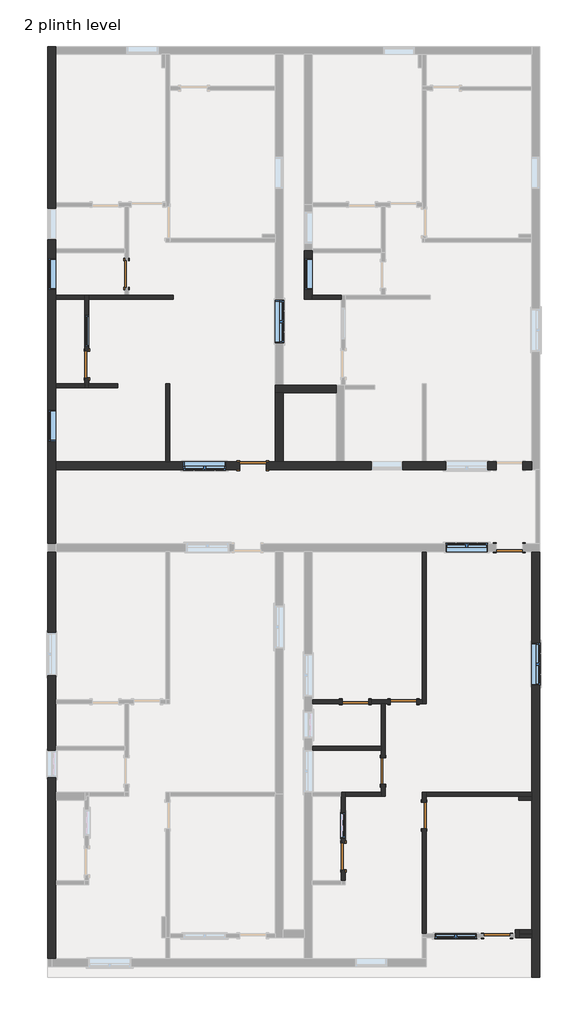
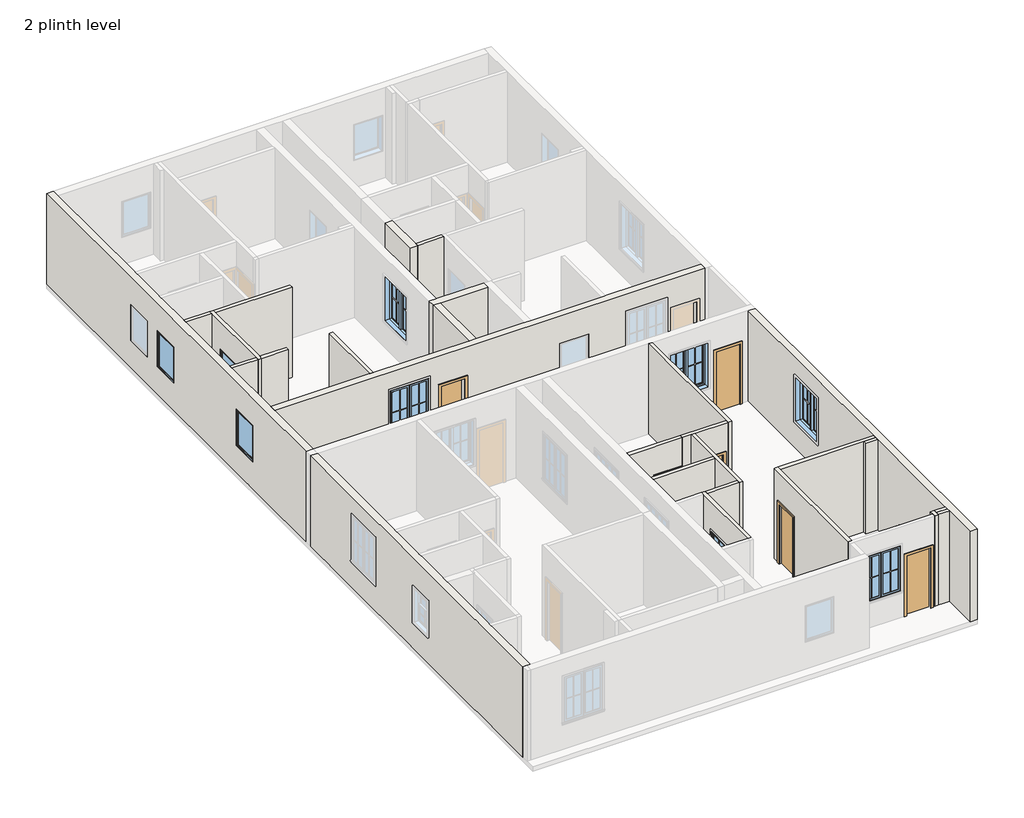
# One storey, part 2 of 4: 27 walls, 10 doors, 10 windows.
"""IFC4 building model written with IfcOpenShell, lengths in millimetres."""

from ifc_helpers import new_model, si_unit, frame, origin, place, context, project, spatial, polyline, outline, extrude, faceted_brep, transform, mapped, element, save
from components import door_d8f5dbb5, door_a1484949, door_f2b275c1, door_85036156, window_c1f32544, window_41a96561, window_8377141f, window_d9d3dda5, window_5a369d27

model = new_model("IFC4")

# Units and contexts
model_context = context("Model", 3, world=origin())
ifc_project = project(units=[si_unit("LENGTHUNIT", "METRE", prefix="MILLI")], contexts=[model_context])

# Site, building, storey
site = spatial("IfcSite", under=ifc_project)
building = spatial("IfcBuilding", under=site)
storey = spatial("IfcBuildingStorey", under=building, Name="2 plinth level", Elevation=457.2)

# Doors
placement = place(None, origin())
door_shape = door_d8f5dbb5(model_context)
element("IfcDoor", 1, ObjectType="Single-Flush : 30\" x 80\"", at=placement, inside=storey, context=model_context, shape_type="MappedRepresentation", body=[
    mapped(door_shape, transform((4590.996455, -11604.0784449, 457.2), x_axis=(1.0, 0.0, 0.0), y_axis=(0.0, 1.0, 0.0), z_axis=(0.0, 0.0, 1.0))),
])
element("IfcDoor", 2, ObjectType="Single-Flush : 30\" x 80\"", at=placement, inside=storey, context=model_context, shape_type="MappedRepresentation", body=[
    mapped(door_shape, transform((1896.0224532, -4857.3304449, 457.2), x_axis=(1.0, 0.0, 0.0), y_axis=(0.0, 1.0, 0.0), z_axis=(0.0, 0.0, 1.0))),
])
door_2_shape = door_a1484949(model_context)
element("IfcDoor", 3, ObjectType="Single-Flush : 30\" x 80\"", at=placement, inside=storey, context=model_context, shape_type="MappedRepresentation", body=[
    mapped(door_2_shape, transform((-2447.3775468, 1943.5195552, 457.2), x_axis=(1.0, 0.0, 0.0), y_axis=(0.0, 1.0, 0.0), z_axis=(0.0, 0.0, 1.0))),
])
door_3_shape = door_f2b275c1(model_context)
element("IfcDoor", 4, ObjectType="Single-Flush : 30\" x 80\"", at=placement, inside=storey, context=model_context, shape_type="MappedRepresentation", body=[
    mapped(door_3_shape, transform((-6085.9275468, 7468.0195551, 457.2), x_axis=(0.0, -1.0, 0.0), y_axis=(1.0, 0.0, 0.0), z_axis=(0.0, 0.0, 1.0))),
])
element("IfcDoor", 5, ObjectType="Single-Flush : 30\" x 80\"", at=placement, inside=storey, context=model_context, shape_type="MappedRepresentation", body=[
    mapped(door_3_shape, transform((-7228.9275468, 4858.1695551, 457.2), x_axis=(0.0, -1.0, 0.0), y_axis=(1.0, 0.0, 0.0), z_axis=(0.0, 0.0, 1.0))),
])
element("IfcDoor", 6, ObjectType="Single-Flush : 30\" x 80\"", at=placement, inside=storey, context=model_context, shape_type="MappedRepresentation", body=[
    mapped(door_3_shape, transform((505.5435023, -4857.3304449, 457.2), x_axis=(1.0, 0.0, 0.0), y_axis=(0.0, 1.0, 0.0), z_axis=(0.0, 0.0, 1.0))),
])
element("IfcDoor", 7, ObjectType="Single-Flush : 30\" x 80\"", at=placement, inside=storey, context=model_context, shape_type="MappedRepresentation", body=[
    mapped(door_3_shape, transform((1305.4724532, -6857.5804449, 457.2), x_axis=(0.0, -1.0, 0.0), y_axis=(1.0, 0.0, 0.0), z_axis=(0.0, 0.0, 1.0))),
])
element("IfcDoor", 8, ObjectType="Single-Flush : 30\" x 80\"", at=placement, inside=storey, context=model_context, shape_type="MappedRepresentation", body=[
    mapped(door_3_shape, transform((162.4724532, -9315.0304449, 457.2), x_axis=(0.0, -1.0, 0.0), y_axis=(1.0, 0.0, 0.0), z_axis=(0.0, 0.0, 1.0))),
])
element("IfcDoor", 9, ObjectType="Single-Flush : 30\" x 80\"", at=placement, inside=storey, context=model_context, shape_type="MappedRepresentation", body=[
    mapped(door_3_shape, transform((2486.5724532, -8133.9304449, 457.2), x_axis=(0.0, 1.0, 0.0), y_axis=(-1.0, 0.0, 0.0), z_axis=(0.0, 0.0, 1.0))),
])
door_4_shape = door_85036156(model_context)
element("IfcDoor", 10, ObjectType="Single-Flush : 30\" x 80\"", at=placement, inside=storey, context=model_context, shape_type="MappedRepresentation", body=[
    mapped(door_4_shape, transform((4944.0224532, -418.6804449, 457.2), x_axis=(1.0, 0.0, 0.0), y_axis=(0.0, 1.0, 0.0), z_axis=(0.0, 0.0, 1.0))),
])

# Walls
element("IfcWall", 11, ObjectType="4.5\"", at=placement, inside=storey, context=model_context, shape_type="SweptSolid", body=[
    extrude(outline(polyline([(-7286.0775468, 6744.1195551), (-8124.2775468, 6744.1195551), (-8124.2775468, 6858.4195551), (-7286.0775468, 6858.4195551), (-7286.0775468, 6744.1195551)])), frame((0.0, 0.0, 457.2), z_axis=(0.0, 0.0, 1.0), x_axis=(1.0, 0.0, 0.0)), (0.0, 0.0, 1.0), 3048.0),
])
element("IfcWall", 12, ObjectType="4.5\"", at=placement, inside=storey, context=model_context, shape_type="Brep", body=[
    faceted_brep([(-7171.7775468, 6744.1195551, 457.2), (-4733.3775468, 6744.1195551, 457.2), (-4733.3775468, 6744.1195551, 3505.2), (-7171.7775468, 6744.1195551, 3505.2), (-7171.7775468, 6858.4195551, 457.2), (-7171.7775468, 6858.4195551, 3505.2), (-6143.0775468, 6858.4195551, 3505.2), (-6028.7775468, 6858.4195551, 3505.2), (-4733.3775468, 6858.4195551, 3505.2), (-4733.3775468, 6858.4195551, 457.2), (-6028.7775468, 6858.4195551, 457.2), (-6143.0775468, 6858.4195551, 457.2)], [[[0, 1, 2, 3]], [[4, 5, 6, 7, 8, 9, 10, 11]], [[1, 0, 4, 11, 10, 9]], [[2, 1, 9, 8]], [[3, 2, 8, 7, 6, 5]], [[0, 3, 5, 4]]]),
])
element("IfcWall", 13, ObjectType="4.5\"", at=placement, inside=storey, context=model_context, shape_type="Brep", body=[
    faceted_brep([(-7171.7775468, 4191.4195551, 457.2), (-7171.7775468, 4305.7195551, 457.2), (-7171.7775468, 4477.1695551, 457.2), (-7171.7775468, 4477.1695551, 2489.2), (-7171.7775468, 5239.1695551, 2489.2), (-7171.7775468, 5239.1695551, 457.2), (-7171.7775468, 6744.1195551, 457.2), (-7171.7775468, 6858.4195551, 457.2), (-7171.7775468, 6858.4195551, 3505.2), (-7171.7775468, 6744.1195551, 3505.2), (-7171.7775468, 4305.7195551, 3505.2), (-7171.7775468, 4191.4195551, 3505.2), (-7171.7775468, 6286.9195551, 2590.8), (-7171.7775468, 6286.9195551, 1371.6), (-7171.7775468, 5372.5195551, 1371.6), (-7171.7775468, 5372.5195551, 2590.8), (-7286.0775468, 4477.1695551, 2489.2), (-7286.0775468, 4477.1695551, 457.2), (-7286.0775468, 4305.7195551, 457.2), (-7286.0775468, 4191.4195551, 457.2), (-7286.0775468, 4191.4195551, 3505.2), (-7286.0775468, 4305.7195551, 3505.2), (-7286.0775468, 6744.1195551, 3505.2), (-7286.0775468, 6858.4195551, 3505.2), (-7286.0775468, 6858.4195551, 457.2), (-7286.0775468, 6744.1195551, 457.2), (-7286.0775468, 5239.1695551, 457.2), (-7286.0775468, 5239.1695551, 2489.2), (-7286.0775468, 6286.9195551, 2590.8), (-7286.0775468, 5372.5195551, 2590.8), (-7286.0775468, 5372.5195551, 1371.6), (-7286.0775468, 6286.9195551, 1371.6)], [[[0, 1, 2, 3, 4, 5, 6, 7, 8, 9, 10, 11], [12, 13, 14, 15]], [[16, 17, 18, 19, 20, 21, 22, 23, 24, 25, 26, 27], [28, 29, 30, 31]], [[19, 18, 17, 2, 1, 0]], [[26, 25, 24, 7, 6, 5]], [[11, 10, 9, 8, 23, 22, 21, 20]], [[8, 7, 24, 23]], [[0, 11, 20, 19]], [[3, 2, 17, 16]], [[4, 3, 16, 27]], [[5, 4, 27, 26]], [[13, 12, 28, 31]], [[14, 13, 31, 30]], [[15, 14, 30, 29]], [[12, 15, 29, 28]]]),
])
element("IfcWall", 14, ObjectType="4.5\"", at=placement, inside=storey, context=model_context, shape_type="SweptSolid", body=[
    extrude(outline(polyline([(-7286.0775468, 4191.4195551), (-8124.2775468, 4191.4195551), (-8124.2775468, 4305.7195551), (-7286.0775468, 4305.7195551), (-7286.0775468, 4191.4195551)])), frame((0.0, 0.0, 457.2), z_axis=(0.0, 0.0, 1.0), x_axis=(1.0, 0.0, 0.0)), (0.0, 0.0, 1.0), 3048.0),
])
element("IfcWall", 15, ObjectType="4.5\"", at=placement, inside=storey, context=model_context, shape_type="SweptSolid", body=[
    extrude(outline(polyline([(-4961.9775468, 2057.8195552), (-4961.9775468, 4305.7195551), (-4847.6775468, 4305.7195551), (-4847.6775468, 2057.8195552), (-4961.9775468, 2057.8195552)])), frame((0.0, 0.0, 457.2), z_axis=(0.0, 0.0, 1.0), x_axis=(1.0, 0.0, 0.0)), (0.0, 0.0, 1.0), 3048.0),
])
element("IfcWall", 16, ObjectType="4.5\"", at=placement, inside=storey, context=model_context, shape_type="SweptSolid", body=[
    extrude(outline(polyline([(105.3224532, 6744.1195551), (-732.8775468, 6744.1195551), (-732.8775468, 6858.4195551), (105.3224532, 6858.4195551), (105.3224532, 6744.1195551)])), frame((0.0, 0.0, 457.2), z_axis=(0.0, 0.0, 1.0), x_axis=(1.0, 0.0, 0.0)), (0.0, 0.0, 1.0), 3048.0),
])
element("IfcWall", 17, ObjectType="4.5\"", at=placement, inside=storey, context=model_context, shape_type="SweptSolid", body=[
    extrude(outline(polyline([(-7171.7775468, 4305.7195551), (-6332.5155352, 4305.7195551), (-6332.5155352, 4191.4195551), (-7171.7775468, 4191.4195551), (-7171.7775468, 4305.7195551)])), frame((0.0, 0.0, 457.2), z_axis=(0.0, 0.0, 1.0), x_axis=(1.0, 0.0, 0.0)), (0.0, 0.0, 1.0), 3048.0),
])
element("IfcWall", 18, ObjectType="4.5\"", at=placement, inside=storey, context=model_context, shape_type="Brep", body=[
    faceted_brep([(2543.7224532, -4914.4804449, 457.2), (2543.7224532, -532.9804449, 457.2), (2543.7224532, -532.9804449, 3505.2), (2543.7224532, -4914.4804449, 3505.2), (2429.4224532, -4914.4804449, 457.2), (2429.4224532, -4914.4804449, 3505.2), (2429.4224532, -4800.1804449, 3505.2), (2429.4224532, -532.9804449, 3505.2), (2429.4224532, -532.9804449, 457.2), (2429.4224532, -4800.1804449, 457.2)], [[[0, 1, 2, 3]], [[4, 5, 6, 7, 8, 9]], [[1, 0, 4, 9, 8]], [[3, 2, 7, 6, 5]], [[2, 1, 8, 7]], [[0, 3, 5, 4]]]),
])
element("IfcWall", 19, ObjectType="4.5\"", at=placement, inside=storey, context=model_context, shape_type="SweptSolid", body=[
    extrude(outline(polyline([(2489.2, 886.5435023), (457.2, 886.5435023), (457.2, 962.7435023), (3505.2, 962.7435023), (3505.2, -732.8775468), (457.2, -732.8775468), (457.2, 124.5435023), (2489.2, 124.5435023), (2489.2, 886.5435023)])), frame((0.0, -4914.4804449, 0.0), z_axis=(0.0, 1.0, 0.0), x_axis=(0.0, 0.0, 1.0)), (0.0, 0.0, 1.0), 114.3),
])
element("IfcWall", 20, ObjectType="4.5\"", at=placement, inside=storey, context=model_context, shape_type="Brep", body=[
    faceted_brep([(1362.6224532, -7581.4804449, 457.2), (1362.6224532, -7238.5804449, 457.2), (1362.6224532, -7238.5804449, 2489.2), (1362.6224532, -6476.5804449, 2489.2), (1362.6224532, -6476.5804449, 457.2), (1362.6224532, -4914.4804449, 457.2), (1362.6224532, -4914.4804449, 3505.2), (1362.6224532, -7581.4804449, 3505.2), (1248.3224532, -7238.5804449, 2489.2), (1248.3224532, -7238.5804449, 457.2), (1248.3224532, -7467.1804449, 457.2), (1248.3224532, -7581.4804449, 457.2), (1248.3224532, -7581.4804449, 3505.2), (1248.3224532, -7467.1804449, 3505.2), (1248.3224532, -6247.9804449, 3505.2), (1248.3224532, -6133.6804449, 3505.2), (1248.3224532, -4914.4804449, 3505.2), (1248.3224532, -4914.4804449, 457.2), (1248.3224532, -6133.6804449, 457.2), (1248.3224532, -6247.9804449, 457.2), (1248.3224532, -6476.5804449, 457.2), (1248.3224532, -6476.5804449, 2489.2)], [[[0, 1, 2, 3, 4, 5, 6, 7]], [[8, 9, 10, 11, 12, 13, 14, 15, 16, 17, 18, 19, 20, 21]], [[11, 10, 9, 1, 0]], [[20, 19, 18, 17, 5, 4]], [[7, 6, 16, 15, 14, 13, 12]], [[6, 5, 17, 16]], [[0, 7, 12, 11]], [[2, 1, 9, 8]], [[3, 2, 8, 21]], [[4, 3, 21, 20]]]),
])
element("IfcWall", 21, ObjectType="4.5\"", at=placement, inside=storey, context=model_context, shape_type="SweptSolid", body=[
    extrude(outline(polyline([(1248.3224532, -6247.9804449), (-732.8775468, -6247.9804449), (-732.8775468, -6133.6804449), (1248.3224532, -6133.6804449), (1248.3224532, -6247.9804449)])), frame((0.0, 0.0, 457.2), z_axis=(0.0, 0.0, 1.0), x_axis=(1.0, 0.0, 0.0)), (0.0, 0.0, 1.0), 3048.0),
])
element("IfcWall", 22, ObjectType="4.5\"", at=placement, inside=storey, context=model_context, shape_type="Brep", body=[
    faceted_brep([(2543.7224532, -7752.9304449, 2489.2), (2543.7224532, -7752.9304449, 457.2), (2543.7224532, -7581.4804449, 457.2), (2543.7224532, -7467.1804449, 457.2), (2543.7224532, -7467.1804449, 3505.2), (2543.7224532, -7581.4804449, 3505.2), (2543.7224532, -11546.9284449, 3505.2), (2543.7224532, -11546.9284449, 457.2), (2543.7224532, -8514.9304449, 457.2), (2543.7224532, -8514.9304449, 2489.2), (2429.4224532, -7467.1804449, 457.2), (2429.4224532, -7752.9304449, 457.2), (2429.4224532, -7752.9304449, 2489.2), (2429.4224532, -8514.9304449, 2489.2), (2429.4224532, -8514.9304449, 457.2), (2429.4224532, -11546.9284449, 457.2), (2429.4224532, -11546.9284449, 3505.2), (2429.4224532, -7467.1804449, 3505.2)], [[[0, 1, 2, 3, 4, 5, 6, 7, 8, 9]], [[10, 11, 12, 13, 14, 15, 16, 17]], [[8, 7, 15, 14]], [[3, 2, 1, 11, 10]], [[6, 5, 4, 17, 16]], [[4, 3, 10, 17]], [[7, 6, 16, 15]], [[12, 11, 1, 0]], [[13, 12, 0, 9]], [[14, 13, 9, 8]]]),
])
element("IfcWall", 23, ObjectType="4.5\"", at=placement, inside=storey, context=model_context, shape_type="SweptSolid", body=[
    extrude(outline(polyline([(1248.3224532, -7581.4804449), (219.6224532, -7581.4804449), (219.6224532, -7467.1804449), (1248.3224532, -7467.1804449), (1248.3224532, -7581.4804449)])), frame((0.0, 0.0, 457.2), z_axis=(0.0, 0.0, 1.0), x_axis=(1.0, 0.0, 0.0)), (0.0, 0.0, 1.0), 3048.0),
])
element("IfcWall", 24, ObjectType="4.5\"", at=placement, inside=storey, context=model_context, shape_type="Brep", body=[
    faceted_brep([(105.3224532, -9696.0304449, 2489.2), (105.3224532, -9696.0304449, 457.2), (105.3224532, -10019.8804449, 457.2), (105.3224532, -10019.8804449, 3505.2), (105.3224532, -7581.4804449, 3505.2), (105.3224532, -7467.1804449, 3505.2), (105.3224532, -7467.1804449, 457.2), (105.3224532, -7581.4804449, 457.2), (105.3224532, -8934.0304449, 457.2), (105.3224532, -8934.0304449, 2489.2), (105.3224532, -8800.6804449, 2540.0), (105.3224532, -8800.6804449, 1371.6), (105.3224532, -8038.6804449, 1371.6), (105.3224532, -8038.6804449, 2540.0), (219.6224532, -10019.8804449, 457.2), (219.6224532, -9696.0304449, 457.2), (219.6224532, -9696.0304449, 2489.2), (219.6224532, -8934.0304449, 2489.2), (219.6224532, -8934.0304449, 457.2), (219.6224532, -7581.4804449, 457.2), (219.6224532, -7467.1804449, 457.2), (219.6224532, -7467.1804449, 3505.2), (219.6224532, -7581.4804449, 3505.2), (219.6224532, -10019.8804449, 3505.2), (219.6224532, -8800.6804449, 2540.0), (219.6224532, -8038.6804449, 2540.0), (219.6224532, -8038.6804449, 1371.6), (219.6224532, -8800.6804449, 1371.6)], [[[0, 1, 2, 3, 4, 5, 6, 7, 8, 9], [10, 11, 12, 13]], [[14, 15, 16, 17, 18, 19, 20, 21, 22, 23], [24, 25, 26, 27]], [[2, 1, 15, 14]], [[8, 7, 6, 20, 19, 18]], [[5, 4, 3, 23, 22, 21]], [[6, 5, 21, 20]], [[3, 2, 14, 23]], [[16, 15, 1, 0]], [[17, 16, 0, 9]], [[18, 17, 9, 8]], [[11, 10, 24, 27]], [[12, 11, 27, 26]], [[13, 12, 26, 25]], [[10, 13, 25, 24]]]),
])
element("IfcWall", 25, ObjectType="4.5\"", at=placement, inside=storey, context=model_context, shape_type="Brep", body=[
    faceted_brep([(2277.0224532, -4914.4804449, 2489.2), (2277.0224532, -4914.4804449, 457.2), (2429.4224532, -4914.4804449, 457.2), (2429.4224532, -4914.4804449, 3505.2), (1362.6224532, -4914.4804449, 3505.2), (1248.3224532, -4914.4804449, 3505.2), (962.7435023, -4914.4804449, 3505.2), (962.7435023, -4914.4804449, 457.2), (1248.3224532, -4914.4804449, 457.2), (1362.6224532, -4914.4804449, 457.2), (1515.0224532, -4914.4804449, 457.2), (1515.0224532, -4914.4804449, 2489.2), (2429.4224532, -4800.1804449, 457.2), (2277.0224532, -4800.1804449, 457.2), (2277.0224532, -4800.1804449, 2489.2), (1515.0224532, -4800.1804449, 2489.2), (1515.0224532, -4800.1804449, 457.2), (962.7435023, -4800.1804449, 457.2), (962.7435023, -4800.1804449, 3505.2), (2429.4224532, -4800.1804449, 3505.2)], [[[0, 1, 2, 3, 4, 5, 6, 7, 8, 9, 10, 11]], [[12, 13, 14, 15, 16, 17, 18, 19]], [[2, 1, 13, 12]], [[10, 9, 8, 7, 17, 16]], [[6, 5, 4, 3, 19, 18]], [[7, 6, 18, 17]], [[3, 2, 12, 19]], [[14, 13, 1, 0]], [[15, 14, 0, 11]], [[16, 15, 11, 10]]]),
])
element("IfcWall", 26, ObjectType="4.5\"", at=placement, inside=storey, context=model_context, shape_type="SweptSolid", body=[
    extrude(outline(polyline([(5591.7224532, -7581.4804449), (2543.7224532, -7581.4804449), (2543.7224532, -7467.1804449), (5591.7224532, -7467.1804449), (5591.7224532, -7581.4804449)])), frame((0.0, 0.0, 457.2), z_axis=(0.0, 0.0, 1.0), x_axis=(1.0, 0.0, 0.0)), (0.0, 0.0, 1.0), 3048.0),
])
element("IfcWall", 27, ObjectType="4.5\"", at=placement, inside=storey, context=model_context, shape_type="SweptSolid", body=[
    extrude(outline(polyline([(3952.7813613, -11546.9284449), (3952.7813613, -11543.8804449), (4067.0813613, -11543.8804449), (4067.0813613, -11546.9284449), (3952.7813613, -11546.9284449)])), frame((0.0, 0.0, 457.2), z_axis=(0.0, 0.0, 1.0), x_axis=(1.0, 0.0, 0.0)), (0.0, 0.0, 1.0), 3048.0),
])
element("IfcWall", 28, ObjectType="4.5\"", at=placement, inside=storey, context=model_context, shape_type="Brep", body=[
    faceted_brep([(5114.9115487, -11429.5804449, 457.2), (5114.9115487, -11546.9284449, 457.2), (5114.9115487, -11661.2284449, 457.2), (5114.9115487, -11661.2284449, 3505.2), (5114.9115487, -11546.9284449, 3505.2), (5114.9115487, -11429.5804449, 3505.2), (5229.2115487, -11429.5804449, 457.2), (5229.2115487, -11429.5804449, 3505.2), (5229.2115487, -11543.8804449, 3505.2), (5229.2115487, -11658.1804449, 3505.2), (5229.2115487, -11661.2284449, 3505.2), (5229.2115487, -11661.2284449, 457.2), (5229.2115487, -11658.1804449, 457.2), (5229.2115487, -11543.8804449, 457.2)], [[[0, 1, 2, 3, 4, 5]], [[6, 7, 8, 9, 10, 11, 12, 13]], [[2, 1, 0, 6, 13, 12, 11]], [[5, 4, 3, 10, 9, 8, 7]], [[0, 5, 7, 6]], [[3, 2, 11, 10]]]),
])
element("IfcWall", 29, ObjectType="4.5\"", at=placement, inside=storey, context=model_context, shape_type="SweptSolid", body=[
    extrude(outline(polyline([(5229.2115487, -11429.5804449), (5591.7224532, -11429.5804449), (5591.7224532, -11543.8804449), (5229.2115487, -11543.8804449), (5229.2115487, -11429.5804449)])), frame((0.0, 0.0, 457.2), z_axis=(0.0, 0.0, 1.0), x_axis=(1.0, 0.0, 0.0)), (0.0, 0.0, 1.0), 3048.0),
])
element("IfcWall", 30, ObjectType="4.5\"", at=placement, inside=storey, context=model_context, shape_type="SweptSolid", body=[
    extrude(outline(polyline([(5591.7224532, -11658.1804449), (5229.2115487, -11658.1804449), (5229.2115487, -11543.8804449), (5591.7224532, -11543.8804449), (5591.7224532, -11658.1804449)])), frame((0.0, 0.0, 457.2), z_axis=(0.0, 0.0, 1.0), x_axis=(1.0, 0.0, 0.0)), (0.0, 0.0, 1.0), 3048.0),
])
element("IfcWall", 31, ObjectType="4.5\"", at=placement, inside=storey, context=model_context, shape_type="SweptSolid", body=[
    extrude(outline(polyline([(5591.7224532, -7695.7804449), (5210.7224532, -7695.7804449), (5210.7224532, -7581.4804449), (5591.7224532, -7581.4804449), (5591.7224532, -7695.7804449)])), frame((0.0, 0.0, 457.2), z_axis=(0.0, 0.0, 1.0), x_axis=(1.0, 0.0, 0.0)), (0.0, 0.0, 1.0), 3048.0),
])
element("IfcWall", 32, ObjectType="9\"", at=placement, inside=storey, context=model_context, shape_type="Brep", body=[
    faceted_brep([(-8352.8775468, 14021.2195551, 457.2), (-8352.8775468, -12267.7804449, 457.2), (-8352.8775468, -12267.7804449, 3505.2), (-8352.8775468, 14021.2195551, 3505.2), (-8352.8775468, 9366.6695551, 2590.8), (-8352.8775468, 8452.2695551, 2590.8), (-8352.8775468, 8452.2695551, 1371.6), (-8352.8775468, 9366.6695551, 1371.6), (-8352.8775468, 3553.2445551, 2590.8), (-8352.8775468, 2638.8445551, 2590.8), (-8352.8775468, 2638.8445551, 1371.6), (-8352.8775468, 3553.2445551, 1371.6), (-8352.8775468, 7925.2195551, 2590.8), (-8352.8775468, 7010.8195551, 2590.8), (-8352.8775468, 7010.8195551, 1371.6), (-8352.8775468, 7925.2195551, 1371.6), (-8352.8775468, -2876.1304449, 2895.6), (-8352.8775468, -4095.3304449, 2895.6), (-8352.8775468, -4095.3304449, 1371.6), (-8352.8775468, -2876.1304449, 1371.6), (-8352.8775468, -6267.0304448, 2540.0), (-8352.8775468, -7029.0304448, 2540.0), (-8352.8775468, -7029.0304448, 1371.6), (-8352.8775468, -6267.0304448, 1371.6), (-8124.2775468, 14021.2195551, 457.2), (-8124.2775468, 14021.2195551, 3505.2), (-8124.2775468, 13792.6195551, 3505.2), (-8124.2775468, 9525.4195551, 3505.2), (-8124.2775468, 9411.1195551, 3505.2), (-8124.2775468, 8191.9195552, 3505.2), (-8124.2775468, 8077.6195552, 3505.2), (-8124.2775468, 6858.4195551, 3505.2), (-8124.2775468, 6744.1195551, 3505.2), (-8124.2775468, 4305.7195551, 3505.2), (-8124.2775468, 4191.4195551, 3505.2), (-8124.2775468, 2057.8195552, 3505.2), (-8124.2775468, 1829.2195552, 3505.2), (-8124.2775468, -4800.1804449, 3505.2), (-8124.2775468, -4914.4804449, 3505.2), (-8124.2775468, -6133.6804448, 3505.2), (-8124.2775468, -6247.9804448, 3505.2), (-8124.2775468, -7467.1804449, 3505.2), (-8124.2775468, -7695.7804449, 3505.2), (-8124.2775468, -10019.8804449, 3505.2), (-8124.2775468, -10134.1804449, 3505.2), (-8124.2775468, -12267.7804449, 3505.2), (-8124.2775468, -12267.7804449, 457.2), (-8124.2775468, -10134.1804449, 457.2), (-8124.2775468, -10019.8804449, 457.2), (-8124.2775468, -7695.7804449, 457.2), (-8124.2775468, -7467.1804449, 457.2), (-8124.2775468, -6247.9804448, 457.2), (-8124.2775468, -6133.6804448, 457.2), (-8124.2775468, -4914.4804449, 457.2), (-8124.2775468, -4800.1804449, 457.2), (-8124.2775468, 1829.2195552, 457.2), (-8124.2775468, 2057.8195552, 457.2), (-8124.2775468, 4191.4195551, 457.2), (-8124.2775468, 4305.7195551, 457.2), (-8124.2775468, 6744.1195551, 457.2), (-8124.2775468, 6858.4195551, 457.2), (-8124.2775468, 8077.6195552, 457.2), (-8124.2775468, 8191.9195552, 457.2), (-8124.2775468, 9411.1195551, 457.2), (-8124.2775468, 9525.4195551, 457.2), (-8124.2775468, 13792.6195551, 457.2), (-8124.2775468, 9366.6695551, 2590.8), (-8124.2775468, 9366.6695551, 1371.6), (-8124.2775468, 8452.2695551, 1371.6), (-8124.2775468, 8452.2695551, 2590.8), (-8124.2775468, 3553.2445551, 2590.8), (-8124.2775468, 3553.2445551, 1371.6), (-8124.2775468, 2638.8445551, 1371.6), (-8124.2775468, 2638.8445551, 2590.8), (-8124.2775468, 7925.2195551, 2590.8), (-8124.2775468, 7925.2195551, 1371.6), (-8124.2775468, 7010.8195551, 1371.6), (-8124.2775468, 7010.8195551, 2590.8), (-8124.2775468, -2876.1304449, 2895.6), (-8124.2775468, -2876.1304449, 1371.6), (-8124.2775468, -4095.3304449, 1371.6), (-8124.2775468, -4095.3304449, 2895.6), (-8124.2775468, -6267.0304448, 2540.0), (-8124.2775468, -6267.0304448, 1371.6), (-8124.2775468, -7029.0304448, 1371.6), (-8124.2775468, -7029.0304448, 2540.0), (-8238.5775468, -12267.7804449, 457.2), (-8238.5775468, -12267.7804449, 3505.2)], [[[0, 1, 2, 3], [4, 5, 6, 7], [8, 9, 10, 11], [12, 13, 14, 15], [16, 17, 18, 19], [20, 21, 22, 23]], [[24, 25, 26, 27, 28, 29, 30, 31, 32, 33, 34, 35, 36, 37, 38, 39, 40, 41, 42, 43, 44, 45, 46, 47, 48, 49, 50, 51, 52, 53, 54, 55, 56, 57, 58, 59, 60, 61, 62, 63, 64, 65], [66, 67, 68, 69], [70, 71, 72, 73], [74, 75, 76, 77], [78, 79, 80, 81], [82, 83, 84, 85]], [[1, 0, 24, 65, 64, 63, 62, 61, 60, 59, 58, 57, 56, 55, 54, 53, 52, 51, 50, 49, 48, 47, 46, 86]], [[3, 2, 87, 45, 44, 43, 42, 41, 40, 39, 38, 37, 36, 35, 34, 33, 32, 31, 30, 29, 28, 27, 26, 25]], [[0, 3, 25, 24]], [[2, 1, 86, 46, 45, 87]], [[67, 66, 4, 7]], [[68, 67, 7, 6]], [[69, 68, 6, 5]], [[66, 69, 5, 4]], [[71, 70, 8, 11]], [[72, 71, 11, 10]], [[73, 72, 10, 9]], [[70, 73, 9, 8]], [[75, 74, 12, 15]], [[76, 75, 15, 14]], [[77, 76, 14, 13]], [[74, 77, 13, 12]], [[79, 78, 16, 19]], [[80, 79, 19, 18]], [[81, 80, 18, 17]], [[78, 81, 17, 16]], [[83, 82, 20, 23]], [[84, 83, 23, 22]], [[85, 84, 22, 21]], [[82, 85, 21, 20]]]),
])
element("IfcWall", 33, ObjectType="9\"", at=placement, inside=storey, context=model_context, shape_type="Brep", body=[
    faceted_brep([(5591.7224532, -532.9804449, 457.2), (5591.7224532, -7467.1804449, 457.2), (5591.7224532, -7581.4804449, 457.2), (5591.7224532, -7695.7804449, 457.2), (5591.7224532, -11429.5804449, 457.2), (5591.7224532, -11543.8804449, 457.2), (5591.7224532, -11658.1804449, 457.2), (5591.7224532, -12801.1804449, 457.2), (5591.7224532, -12801.1804449, 3505.2), (5591.7224532, -11658.1804449, 3505.2), (5591.7224532, -11543.8804449, 3505.2), (5591.7224532, -11429.5804449, 3505.2), (5591.7224532, -7695.7804449, 3505.2), (5591.7224532, -7581.4804449, 3505.2), (5591.7224532, -7467.1804449, 3505.2), (5591.7224532, -532.9804449, 3505.2), (5591.7224532, -4381.0804449, 2895.6), (5591.7224532, -4381.0804449, 1371.6), (5591.7224532, -3161.8804449, 1371.6), (5591.7224532, -3161.8804449, 2895.6), (5820.3224532, -532.9804449, 457.2), (5820.3224532, -532.9804449, 3505.2), (5820.3224532, -12801.1804449, 3505.2), (5820.3224532, -12801.1804449, 457.2), (5820.3224532, -4381.0804449, 2895.6), (5820.3224532, -3161.8804449, 2895.6), (5820.3224532, -3161.8804449, 1371.6), (5820.3224532, -4381.0804449, 1371.6)], [[[0, 1, 2, 3, 4, 5, 6, 7, 8, 9, 10, 11, 12, 13, 14, 15], [16, 17, 18, 19]], [[20, 21, 22, 23], [24, 25, 26, 27]], [[7, 6, 5, 4, 3, 2, 1, 0, 20, 23]], [[8, 7, 23, 22]], [[15, 14, 13, 12, 11, 10, 9, 8, 22, 21]], [[0, 15, 21, 20]], [[17, 16, 24, 27]], [[18, 17, 27, 26]], [[19, 18, 26, 25]], [[16, 19, 25, 24]]]),
])
element("IfcWall", 34, ObjectType="9\"", at=placement, inside=storey, context=model_context, shape_type="SweptSolid", body=[
    extrude(outline(polyline([(-1799.6775468, 2057.8195552), (-1799.6775468, 4039.0195551), (-1571.0775468, 4039.0195551), (-1571.0775468, 2057.8195552), (-1799.6775468, 2057.8195552)])), frame((0.0, 0.0, 457.2), z_axis=(0.0, 0.0, 1.0), x_axis=(1.0, 0.0, 0.0)), (0.0, 0.0, 1.0), 3048.0),
])
element("IfcWall", 35, ObjectType="9\"", at=placement, inside=storey, context=model_context, shape_type="Brep", body=[
    faceted_brep([(5591.7224532, 2057.8195552, 457.2), (5325.0224532, 2057.8195552, 457.2), (5325.0224532, 2057.8195552, 2489.2), (4563.0224532, 2057.8195552, 2489.2), (4563.0224532, 2057.8195552, 457.2), (2543.7224532, 2057.8195552, 457.2), (2429.4224532, 2057.8195552, 457.2), (181.5224532, 2057.8195552, 457.2), (-47.0775468, 2057.8195552, 457.2), (-1571.0775468, 2057.8195552, 457.2), (-1799.6775468, 2057.8195552, 457.2), (-2066.3775468, 2057.8195552, 457.2), (-2066.3775468, 2057.8195552, 2489.2), (-2828.3775468, 2057.8195552, 2489.2), (-2828.3775468, 2057.8195552, 457.2), (-4847.6775468, 2057.8195552, 457.2), (-4961.9775468, 2057.8195552, 457.2), (-8124.2775468, 2057.8195552, 457.2), (-8124.2775468, 2057.8195552, 3505.2), (-4961.9775468, 2057.8195552, 3505.2), (-4847.6775468, 2057.8195552, 3505.2), (-1799.6775468, 2057.8195552, 3505.2), (-1571.0775468, 2057.8195552, 3505.2), (-47.0775468, 2057.8195552, 3505.2), (181.5224532, 2057.8195552, 3505.2), (2429.4224532, 2057.8195552, 3505.2), (2543.7224532, 2057.8195552, 3505.2), (5591.7224532, 2057.8195552, 3505.2), (962.5724532, 2057.8195552, 2590.8), (962.5724532, 2057.8195552, 1371.6), (1876.9724532, 2057.8195552, 1371.6), (1876.9724532, 2057.8195552, 2590.8), (-4447.6275468, 2057.8195552, 2895.6), (-4447.6275468, 2057.8195552, 1371.6), (-3228.4275468, 2057.8195552, 1371.6), (-3228.4275468, 2057.8195552, 2895.6), (3105.6974532, 2057.8195552, 2895.6), (3105.6974532, 2057.8195552, 1371.6), (4324.8974532, 2057.8195552, 1371.6), (4324.8974532, 2057.8195552, 2895.6), (5325.0224532, 1829.2195552, 2489.2), (5325.0224532, 1829.2195552, 457.2), (5591.7224532, 1829.2195552, 457.2), (5591.7224532, 1829.2195552, 3505.2), (-8124.2775468, 1829.2195552, 3505.2), (-8124.2775468, 1829.2195552, 457.2), (-2828.3775468, 1829.2195552, 457.2), (-2828.3775468, 1829.2195552, 2489.2), (-2066.3775468, 1829.2195552, 2489.2), (-2066.3775468, 1829.2195552, 457.2), (4563.0224532, 1829.2195552, 457.2), (4563.0224532, 1829.2195552, 2489.2), (962.5724532, 1829.2195552, 2590.8), (1876.9724532, 1829.2195552, 2590.8), (1876.9724532, 1829.2195552, 1371.6), (962.5724532, 1829.2195552, 1371.6), (-4447.6275468, 1829.2195552, 2895.6), (-3228.4275468, 1829.2195552, 2895.6), (-3228.4275468, 1829.2195552, 1371.6), (-4447.6275468, 1829.2195552, 1371.6), (3105.6974532, 1829.2195552, 2895.6), (4324.8974532, 1829.2195552, 2895.6), (4324.8974532, 1829.2195552, 1371.6), (3105.6974532, 1829.2195552, 1371.6)], [[[0, 1, 2, 3, 4, 5, 6, 7, 8, 9, 10, 11, 12, 13, 14, 15, 16, 17, 18, 19, 20, 21, 22, 23, 24, 25, 26, 27], [28, 29, 30, 31], [32, 33, 34, 35], [36, 37, 38, 39]], [[40, 41, 42, 43, 44, 45, 46, 47, 48, 49, 50, 51], [52, 53, 54, 55], [56, 57, 58, 59], [60, 61, 62, 63]], [[46, 45, 17, 16, 15, 14]], [[50, 49, 11, 10, 9, 8, 7, 6, 5, 4]], [[42, 41, 1, 0]], [[27, 26, 25, 24, 23, 22, 21, 20, 19, 18, 44, 43]], [[18, 17, 45, 44]], [[0, 27, 43, 42]], [[12, 11, 49, 48]], [[13, 12, 48, 47]], [[14, 13, 47, 46]], [[2, 1, 41, 40]], [[3, 2, 40, 51]], [[4, 3, 51, 50]], [[29, 28, 52, 55]], [[30, 29, 55, 54]], [[31, 30, 54, 53]], [[28, 31, 53, 52]], [[33, 32, 56, 59]], [[34, 33, 59, 58]], [[35, 34, 58, 57]], [[32, 35, 57, 56]], [[37, 36, 60, 63]], [[38, 37, 63, 62]], [[39, 38, 62, 61]], [[36, 39, 61, 60]]]),
])
element("IfcWall", 36, ObjectType="9\"", at=placement, inside=storey, context=model_context, shape_type="Brep", body=[
    faceted_brep([(-47.0775468, 4267.6195551, 457.2), (-1571.0775468, 4267.6195551, 457.2), (-1799.6775468, 4267.6195551, 457.2), (-1799.6775468, 4267.6195551, 3505.2), (-1571.0775468, 4267.6195551, 3505.2), (-47.0775468, 4267.6195551, 3505.2), (-47.0775468, 4039.0195551, 457.2), (-47.0775468, 4039.0195551, 3505.2), (-1571.0775468, 4039.0195551, 3505.2), (-1799.6775468, 4039.0195551, 3505.2), (-1799.6775468, 4039.0195551, 457.2), (-1571.0775468, 4039.0195551, 457.2)], [[[0, 1, 2, 3, 4, 5]], [[6, 7, 8, 9, 10, 11]], [[2, 1, 0, 6, 11, 10]], [[5, 4, 3, 9, 8, 7]], [[0, 5, 7, 6]], [[3, 2, 10, 9]]]),
])
element("IfcWall", 37, ObjectType="9\"", at=placement, inside=storey, context=model_context, shape_type="Brep", body=[
    faceted_brep([(-961.4775468, 8134.7695551, 457.2), (-961.4775468, 6744.1195551, 457.2), (-961.4775468, 6744.1195551, 3505.2), (-961.4775468, 8134.7695551, 3505.2), (-961.4775468, 7925.2195551, 2590.8), (-961.4775468, 7010.8195551, 2590.8), (-961.4775468, 7010.8195551, 1371.6), (-961.4775468, 7925.2195551, 1371.6), (-732.8775468, 8134.7695551, 457.2), (-732.8775468, 8134.7695551, 3505.2), (-732.8775468, 8077.6195551, 3505.2), (-732.8775468, 6858.4195551, 3505.2), (-732.8775468, 6744.1195551, 3505.2), (-732.8775468, 6744.1195551, 457.2), (-732.8775468, 6858.4195551, 457.2), (-732.8775468, 8077.6195551, 457.2), (-732.8775468, 7925.2195551, 2590.8), (-732.8775468, 7925.2195551, 1371.6), (-732.8775468, 7010.8195551, 1371.6), (-732.8775468, 7010.8195551, 2590.8)], [[[0, 1, 2, 3], [4, 5, 6, 7]], [[8, 9, 10, 11, 12, 13, 14, 15], [16, 17, 18, 19]], [[1, 0, 8, 15, 14, 13]], [[3, 2, 12, 11, 10, 9]], [[0, 3, 9, 8]], [[2, 1, 13, 12]], [[17, 16, 4, 7]], [[18, 17, 7, 6]], [[19, 18, 6, 5]], [[16, 19, 5, 4]]]),
])

# Windows
window_shape = window_c1f32544(model_context)
element("IfcWindow", 38, ObjectType="Fixed : 36\" x 48\"", at=placement, inside=storey, context=model_context, shape_type="MappedRepresentation", body=[
    mapped(window_shape, transform((-847.1775468, 7506.1195551, 457.2), x_axis=(0.0, 1.0, 0.0), y_axis=(-1.0, 0.0, 0.0), z_axis=(0.0, 0.0, 1.0))),
])
element("IfcWindow", 39, ObjectType="Fixed : 36\" x 48\"", at=placement, inside=storey, context=model_context, shape_type="MappedRepresentation", body=[
    mapped(window_shape, transform((-8238.5775468, 3134.1445551, 457.2), x_axis=(0.0, 1.0, 0.0), y_axis=(-1.0, 0.0, 0.0), z_axis=(0.0, 0.0, 1.0))),
])
element("IfcWindow", 40, ObjectType="Fixed : 36\" x 48\"", at=placement, inside=storey, context=model_context, shape_type="MappedRepresentation", body=[
    mapped(window_shape, transform((-8238.5775468, 7506.1195551, 457.2), x_axis=(0.0, 1.0, 0.0), y_axis=(-1.0, 0.0, 0.0), z_axis=(0.0, 0.0, 1.0))),
])
window_2_shape = window_41a96561(model_context)
element("IfcWindow", 41, ObjectType="Fixed : 36\" x 48\"", at=placement, inside=storey, context=model_context, shape_type="MappedRepresentation", body=[
    mapped(window_2_shape, transform((-7228.9275468, 5867.8195551, 457.2), x_axis=(0.0, 1.0, 0.0), y_axis=(-1.0, 0.0, 0.0), z_axis=(0.0, 0.0, 1.0))),
])
window_3_shape = window_8377141f(model_context)
element("IfcWindow", 42, ObjectType="Window-Casement-Double : 48\" x 60\"", at=placement, inside=storey, context=model_context, shape_type="MappedRepresentation", body=[
    mapped(window_3_shape, transform((3715.2974532, -418.6804449, 457.2), x_axis=(1.0, 0.0, 0.0), y_axis=(0.0, 1.0, 0.0), z_axis=(0.0, 0.0, 1.0))),
])
element("IfcWindow", 43, ObjectType="Window-Casement-Double : 48\" x 60\"", at=placement, inside=storey, context=model_context, shape_type="MappedRepresentation", body=[
    mapped(window_3_shape, transform((5706.0224532, -3771.4804449, 457.2), x_axis=(0.0, -1.0, 0.0), y_axis=(1.0, 0.0, 0.0), z_axis=(0.0, 0.0, 1.0))),
])
element("IfcWindow", 44, ObjectType="Window-Casement-Double : 48\" x 60\"", at=placement, inside=storey, context=model_context, shape_type="MappedRepresentation", body=[
    mapped(window_3_shape, transform((-3838.0275468, 1943.5195552, 457.2), x_axis=(-1.0, 0.0, 0.0), y_axis=(0.0, -1.0, 0.0), z_axis=(0.0, 0.0, 1.0))),
])
element("IfcWindow", 45, ObjectType="Window-Casement-Double : 48\" x 60\"", at=placement, inside=storey, context=model_context, shape_type="MappedRepresentation", body=[
    mapped(window_3_shape, transform((-1685.3775468, 6096.4195551, 457.2), x_axis=(0.0, -1.0, 0.0), y_axis=(1.0, 0.0, 0.0), z_axis=(0.0, 0.0, 1.0))),
])
window_4_shape = window_d9d3dda5(model_context)
element("IfcWindow", 46, ObjectType="Window-Casement-Double : 48\" x 60\"", at=placement, inside=storey, context=model_context, shape_type="MappedRepresentation", body=[
    mapped(window_4_shape, transform((3400.3313613, -11604.0784449, 457.2), x_axis=(-1.0, 0.0, 0.0), y_axis=(0.0, -1.0, 0.0), z_axis=(0.0, 0.0, 1.0))),
])
window_5_shape = window_5a369d27(model_context)
element("IfcWindow", 47, ObjectType="Window-Double-Hung : 30\" x 46\"", at=placement, inside=storey, context=model_context, shape_type="MappedRepresentation", body=[
    mapped(window_5_shape, transform((162.4724532, -8419.6804449, 457.2), x_axis=(0.0, 1.0, 0.0), y_axis=(-1.0, 0.0, 0.0), z_axis=(0.0, 0.0, 1.0))),
])

save(model, "model.ifc")

# Revit data of these elements
# Type "Single-Flush : 30\" x 80\""
#   Type Mark = "5"
#   Construction Type Id = "MDOOR"
#   Assembly Code = "C1020"
#   Analytic Construction = "Metal"
#   Thickness = 0' - 2"
#   Heat Transfer Coefficient (U) = 0.651978 BTU/(h·ft²·°F)
#   Height = 6' - 8"
#   Trim Projection Ext = 0' - 1"
#   Trim Projection Int = 0' - 1"
#   Trim Width = 0' - 3"
#   Width = 2' - 6"
#   Define Thermal Properties by = 1
#   Define Thermal Properties by = 1
#   Door Material = Door - Panel
#   Frame Material = Door - Frame
#   Visual Light Transmittance = 0
#   Solar Heat Gain Coefficient = 0
#   Function = (empty or 0)
#   Wall Closure = (empty or 0)
# Type "4.5\""
#   Assembly Code = "B2010"
#   Layers, outside or top first: 0' - 4 1/2" no material (function 1)
# Type "9\""
#   Assembly Code = "B2010"
#   Layers, outside or top first: 0' - 9" no material (function 1)
# Type "Fixed : 36\" x 48\""
#   Type Mark = "1"
#   Construction Type Id = "GSP4R"
#   Assembly Code = "B2020100"
#   Analytic Construction = "1/8 in Pilkington single glazing"
#   Visual Light Transmittance = 0.9
#   Solar Heat Gain Coefficient = 0.78
#   Heat Transfer Coefficient (U) = 0.6496 BTU/(h·ft²·°F)
#   Height = 4' - 0"
#   Default Sill Height = 3' - 0"
#   Width = 3' - 0"
#   Window Inset = 0' - 0 3/4"
#   Define Thermal Properties by = 1
#   Define Thermal Properties by = 1
#   Glass Pane Material = Glass
#   Sash Material = Sash
#   Wall Closure = (empty or 0)
# Type "Window-Casement-Double : 48\" x 60\""
#   Type Mark = "16"
#   Fire Rating = "0.5h"
#   Assembly Code = "B2020100"
#   Analytic Construction = "Double glazing - domestic"
#   Frame Extension [instance default] = 0' - 0 1/4"
#   Window Inset [instance default] = 0' - 0"
#   Wall Thickness [instance default] = 0' - 6"
#   Interior Wall Closure [instance default] = 0' - 2 1/4"
#   Half Width = 2' - 0"
#   Visual Light Transmittance = 0.81
#   Thermal Resistance (R) = 1.8146 (h·ft²·°F)/BTU
#   Solar Heat Gain Coefficient = 0.76
#   Rough Width = 4' - 0 1/2"
#   Rough Height = 5' - 0 1/2"
#   Height = 5' - 0"
#   Heat Transfer Coefficient (U) = 0.5511 BTU/(h·ft²·°F)
#   Exterior Wall Closure [instance default] = 0' - 1 1/4"
#   Extension Jamb [instance default] = 0' - 2 1/4"
#   Default Sill Height = 3' - 0"
#   Width = 4' - 0"
#   Define Thermal Properties by = 0
#   Muntin Visibility = yes
#   Interior Trim Visibility [instance default] = yes
#   Exterior Trim Visibility [instance default] = yes
#   Extension Jamb Visibility [instance default] = yes
#   Interior Trim Material = Wood - Stained
#   Muntin Pattern = Muntin Pattern_2x2 : Muntin Pattern_2x2
#   Interior Trim = Trim-Window-Interior-Flat : Picture Frame
#   Interior Frame Material = Wood - Stained
#   Glass Panel Material = Glass
#   Exterior Trim Material = Clad - White
#   Exterior Trim = Trim-Window-Exterior-Flat : with Sill
#   Exterior Frame Material = Clad - White
#   Wall Closure = (empty or 0)
# Type "Window-Double-Hung : 30\" x 46\""
#   Type Mark = "13"
#   Fire Rating = "0.5h"
#   Construction Type Id = "DG-DR"
#   Assembly Code = "B2020100"
#   Analytic Construction = "Double glazing - domestic"
#   Wall Thickness [instance default] = 0' - 6"
#   Window Inset [instance default] = 0' - 0"
#   Visual Light Transmittance = 0.81
#   Thermal Resistance (R) = 1.8146 (h·ft²·°F)/BTU
#   Solar Heat Gain Coefficient = 0.76
#   Muntin Width = 2' - 0"
#   Muntin Height = 1' - 7 1/8"
#   Interior Wall Closure [instance default] = 0' - 1 1/2"
#   Rough Width = 2' - 6 1/2"
#   Rough Height = 3' - 10 1/2"
#   Frame Extension [instance default] = 0' - 1 1/4"
#   Exterior Wall Closure [instance default] = 0' - 0 1/2"
#   Extension Jamb [instance default] = 0' - 1 1/2"
#   Heat Transfer Coefficient (U) = 0.5511 BTU/(h·ft²·°F)
#   Height = 3' - 10"
#   Width = 2' - 6"
#   Define Thermal Properties by = 1
#   Top Muntin Visibility = yes
#   Indicator Visibility [instance default] = yes
#   Extension Jamb Visibility [instance default] = yes
#   Interior Trim Visibility [instance default] = yes
#   Exterior Trim Visibility [instance default] = yes
#   Define Thermal Properties by = 1
#   Bottom Muntin Visibility = yes
#   Muntin Pattern = Muntin Pattern_2x2 : Muntin Pattern_2x2
#   Interior Trim Material = Wood - Stained
#   Interior Trim = Trim-Window-Interior-Flat : Picture Frame
#   Exterior Trim Material = Clad - White
#   Exterior Trim = Trim-Window-Exterior-Flat : with Sill
#   Glass Panel Material = Glass
#   Exterior Frame Material = Clad - White
#   Interior Frame Material = Wood - Stained
#   Wall Closure = (empty or 0)
# Elements 1, 2, 3, 4, 5, 6, 7, 8, 9, 10 (IfcDoor, "Single-Flush : 30\" x 80\"")
#   Phase Created = New Construction
#   Materials on its faces: "Door - Frame", "Door - Panel"
# Elements 11, 12, 13, 14, 15, 16, 17, 18, 19, 20, 21, 22, 23, 24, 25, 26, 27, 28, 29, 30, 31 (IfcWall, "4.5\"")
#   Top Offset = 0' - 0"
#   Base Offset = 0' - 0"
#   wall height = 10' - 0"
#   Phase Created = New Construction
#   Base Constraint = 2 plinth level
#   Top Constraint = 3 wall level
#   Materials on its faces: "Default Wall"
# Elements 32, 33, 34, 35, 36, 37 (IfcWall, "9\"")
#   Top Offset = 0' - 0"
#   Base Offset = 0' - 0"
#   wall height = 10' - 0"
#   Phase Created = New Construction
#   Base Constraint = 2 plinth level
#   Top Constraint = 3 wall level
#   Materials on its faces: "Default Wall"
# Element 38 (IfcWindow, "Fixed : 36\" x 48\"")
#   Mark = "15"
#   Phase Created = New Construction
#   Materials on its faces: "Sash", "Glass"
# Element 39 (IfcWindow, "Fixed : 36\" x 48\"")
#   Mark = "18"
#   Phase Created = New Construction
#   Materials on its faces: "Sash", "Glass"
# Element 40 (IfcWindow, "Fixed : 36\" x 48\"")
#   Mark = "19"
#   Phase Created = New Construction
#   Materials on its faces: "Sash", "Glass"
# Element 41 (IfcWindow, "Fixed : 36\" x 48\"")
#   Mark = "20"
#   Phase Created = New Construction
#   Materials on its faces: "Sash", "Glass"
# Element 42 (IfcWindow, "Window-Casement-Double : 48\" x 60\"")
#   Mark = "25"
#   Window Inset = 0' - 0"
#   Interior Wall Closure = 0' - 2 1/4"
#   Frame Extension = 0' - 0 1/4"
#   Exterior Wall Closure = 0' - 1 1/4"
#   Interior Trim Visibility = yes
#   Exterior Trim Visibility = yes
#   Phase Created = New Construction
#   Materials on its faces: "Wood - Stained", "Glass", "Clad - White"
# Element 43 (IfcWindow, "Window-Casement-Double : 48\" x 60\"")
#   Mark = "26"
#   Window Inset = 0' - 0"
#   Interior Wall Closure = 0' - 2 1/4"
#   Frame Extension = 0' - 0 1/4"
#   Exterior Wall Closure = 0' - 1 1/4"
#   Interior Trim Visibility = yes
#   Exterior Trim Visibility = yes
#   Phase Created = New Construction
#   Materials on its faces: "Wood - Stained", "Glass", "Clad - White"
# Element 44 (IfcWindow, "Window-Casement-Double : 48\" x 60\"")
#   Mark = "30"
#   Window Inset = 0' - 0"
#   Interior Wall Closure = 0' - 2 1/4"
#   Frame Extension = 0' - 0 1/4"
#   Exterior Wall Closure = 0' - 1 1/4"
#   Interior Trim Visibility = yes
#   Exterior Trim Visibility = yes
#   Phase Created = New Construction
#   Materials on its faces: "Wood - Stained", "Glass", "Clad - White"
# Element 45 (IfcWindow, "Window-Casement-Double : 48\" x 60\"")
#   Mark = "33"
#   Window Inset = 0' - 0"
#   Interior Wall Closure = 0' - 2 1/4"
#   Frame Extension = 0' - 0 1/4"
#   Exterior Wall Closure = 0' - 1 1/4"
#   Interior Trim Visibility = yes
#   Exterior Trim Visibility = yes
#   Phase Created = New Construction
#   Materials on its faces: "Wood - Stained", "Glass", "Clad - White"
# Element 46 (IfcWindow, "Window-Casement-Double : 48\" x 60\"")
#   Mark = "38"
#   Window Inset = 0' - 0"
#   Interior Wall Closure = 0' - 2 1/4"
#   Frame Extension = 0' - 0 1/4"
#   Exterior Wall Closure = 0' - 1 1/4"
#   Interior Trim Visibility = yes
#   Exterior Trim Visibility = yes
#   Phase Created = New Construction
#   Materials on its faces: "Wood - Stained", "Glass", "Clad - White"
# Element 47 (IfcWindow, "Window-Double-Hung : 30\" x 46\"")
#   Mark = "42"
#   Window Inset = 0' - 0"
#   Interior Wall Closure = 0' - 1 1/2"
#   Frame Extension = 0' - 1 1/4"
#   Exterior Wall Closure = 0' - 0 1/2"
#   Interior Trim Visibility = yes
#   Indicator Visibility = yes
#   Exterior Trim Visibility = yes
#   Phase Created = New Construction
#   Materials on its faces: "Wood - Stained", "Glass", "Clad - White"
# Materials
#   "Door - Panel": class "Wood", colour RGB 210 159 95, transparency 0, Cost = 0
#   "Door - Frame": colour RGB 118 70 51, transparency 0, Cost = 0
#   "Glass": class "Glass", colour RGB 0 128 192, transparency 0.75, Description = "Soda Lime Glass", Cost = 0
#   "Sash": class "Wood", colour RGB 224 178 126, transparency 0, Cost = 0
#   "Wood - Stained": class "Wood", colour RGB 224 178 126, transparency 0, Cost = 0
#   "Clad - White": class "Wood", colour RGB 242 242 238, transparency 0, Cost = 0
#   "Default Wall": colour RGB 128 128 128, transparency 0, Cost = 0
